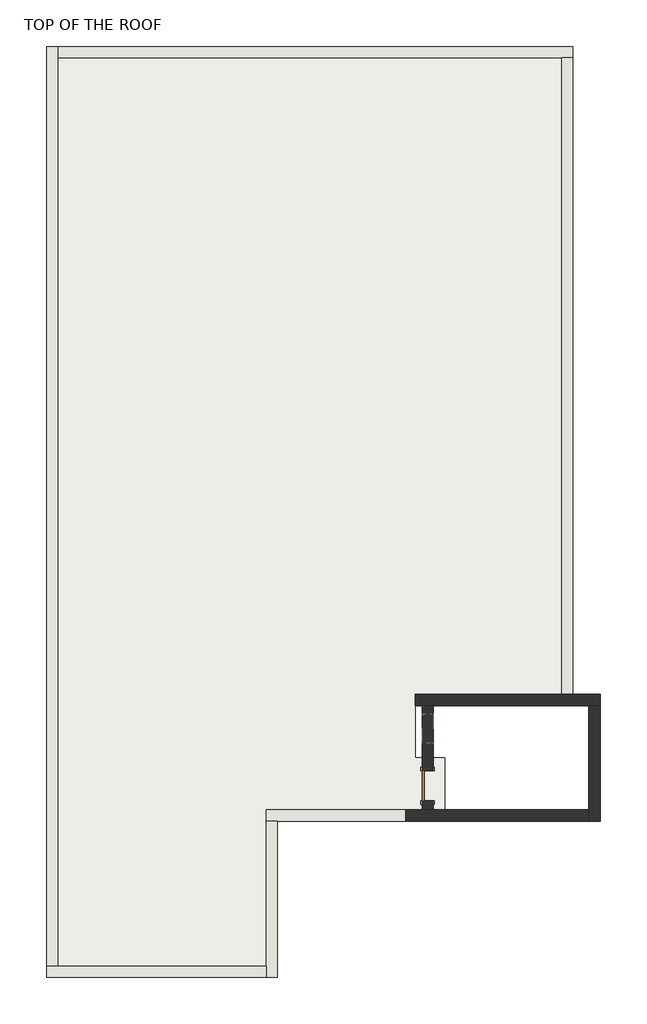
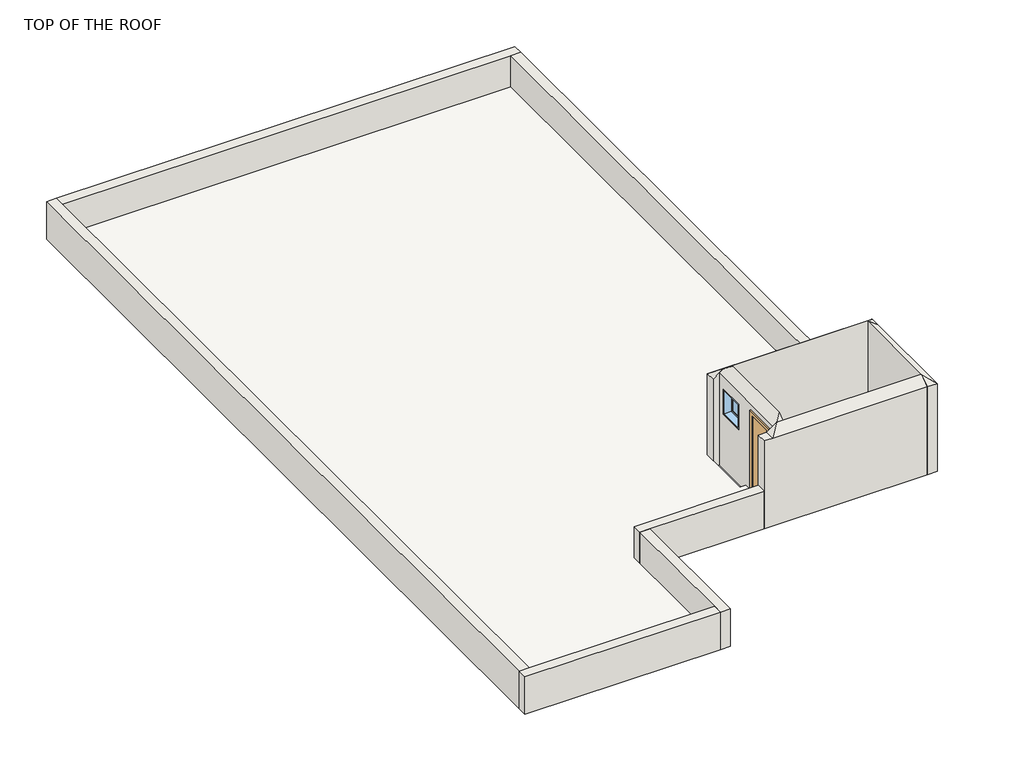
# One storey, incomplete: 10 walls, 1 door, 1 roof, 1 window.
"""IFC4 building model written with IfcOpenShell, lengths in millimetres."""

from ifc_helpers import new_model, si_unit, frame, origin, place, context, project, spatial, polyline, outline, extrude, faceted_brep, transform, mapped, element, save
from components import single_flush_bathroom_flush_door_2_x_7_88cc3d71, window_80340324

model = new_model("IFC4")

# Units and contexts
model_context = context("Model", 3, world=origin())
ifc_project = project(units=[si_unit("LENGTHUNIT", "METRE", prefix="MILLI")], contexts=[model_context])

# Site, building, storey
site = spatial("IfcSite", under=ifc_project)
building = spatial("IfcBuilding", under=site)
storey = spatial("IfcBuildingStorey", under=building, Name="TOP OF THE ROOF", Elevation=6400.8)

# Door
placement = place(None, origin())
single_flush_bathroom_flush_door_2_x_7_shape = single_flush_bathroom_flush_door_2_x_7_88cc3d71(model_context)
element("IfcDoor", 1, ObjectType="Single-Flush : BATHROOM FLUSH DOOR 2' X 7'", at=placement, inside=storey, context=model_context, shape_type="MappedRepresentation", body=[
    mapped(single_flush_bathroom_flush_door_2_x_7_shape, transform((-12501.7436606, -3516.6024127, 6400.8), x_axis=(0.0, 1.0, 0.0), y_axis=(-1.0, 0.0, 0.0), z_axis=(0.0, 0.0, 1.0))),
])

# Roof
element("IfcRoof", 2, ObjectType="Generic - 12\"", at=placement, inside=storey, context=model_context, shape_type="SweptSolid", body=[
    extrude(outline(polyline([(-20070.9436606, 11380.4975873), (-9758.5436606, 11380.4975873), (-9758.5436606, -1649.7024127), (-12755.7436606, -1649.7024127), (-12755.7436606, -1878.3024127), (-12755.7436606, -2945.1024127), (-12146.1436606, -2945.1024127), (-12146.1436606, -4011.9024127), (-15803.7436606, -4011.9024127), (-15803.7436606, -7212.3024127), (-20070.9436606, -7212.3024127), (-20070.9436606, 11380.4975873)])), frame((0.0, 0.0, 6400.8), z_axis=(0.0, 0.0, 1.0), x_axis=(1.0, 0.0, 0.0)), (0.0, 0.0, 1.0), 152.4),
])

# Walls
element("IfcWall", 3, at=placement, inside=storey, context=model_context, shape_type="Brep", body=[
    faceted_brep([(-12755.7436606, -1878.3024127, 6400.8), (-12616.0436606, -1878.3024127, 6400.8), (-12387.4436606, -1878.3024127, 6400.8), (-9199.7436606, -1878.3024127, 6400.8), (-8971.1436606, -1878.3024127, 6400.8), (-8971.1436606, -1878.3024127, 8534.4), (-9199.7436606, -1878.3024127, 8705.85), (-12387.4436606, -1878.3024127, 8705.85), (-12527.1436606, -1878.3024127, 8705.85), (-12616.0436606, -1878.3024127, 8639.175), (-12755.7436606, -1878.3024127, 8534.4), (-12755.7436606, -1649.7024127, 6400.8), (-12755.7436606, -1649.7024127, 8534.4), (-8971.1436606, -1649.7024127, 8534.4), (-8971.1436606, -1649.7024127, 6400.8), (-9529.9436606, -1649.7024127, 6400.8), (-9758.5436606, -1649.7024127, 6400.8)], [[[0, 1, 2, 3, 4, 5, 6, 7, 8, 9, 10]], [[11, 12, 13, 14, 15, 16]], [[4, 3, 2, 1, 0, 11, 16, 15, 14]], [[0, 10, 12, 11]], [[5, 4, 14, 13]], [[10, 9, 8, 12]], [[8, 7, 6, 13, 12]], [[6, 5, 13]]]),
])
element("IfcWall", 4, at=placement, inside=storey, context=model_context, shape_type="Brep", body=[
    faceted_brep([(-9199.7436606, -1878.3024127, 6400.8), (-9199.7436606, -4011.9024127, 6400.8), (-9199.7436606, -4240.5024127, 6400.8), (-9199.7436606, -4240.5024127, 8534.4), (-9199.7436606, -4011.9024127, 8705.85), (-9199.7436606, -1878.3024127, 8705.85), (-8971.1436606, -1878.3024127, 6400.8), (-8971.1436606, -1878.3024127, 8534.4), (-8971.1436606, -4240.5024127, 8534.4), (-8971.1436606, -4240.5024127, 6400.8)], [[[0, 1, 2, 3, 4, 5]], [[6, 7, 8, 9]], [[2, 1, 0, 6, 9]], [[0, 5, 7, 6]], [[3, 2, 9, 8]], [[5, 4, 8, 7]], [[4, 3, 8]]]),
])
element("IfcWall", 5, at=placement, inside=storey, context=model_context, shape_type="Brep", body=[
    faceted_brep([(-9199.7436606, -4011.9024127, 6400.8), (-12387.4436606, -4011.9024127, 6400.8), (-12616.0436606, -4011.9024127, 6400.8), (-12946.2436606, -4011.9024127, 6400.8), (-12946.2436606, -4011.9024127, 7315.2), (-12946.2436606, -4011.9024127, 8534.4), (-12755.7436606, -4011.9024127, 8534.4), (-12616.0436606, -4011.9024127, 8639.175), (-12527.1436606, -4011.9024127, 8705.85), (-12387.4436606, -4011.9024127, 8705.85), (-9199.7436606, -4011.9024127, 8705.85), (-9199.7436606, -4240.5024127, 6400.8), (-9199.7436606, -4240.5024127, 8534.4), (-12755.7436606, -4240.5024127, 8534.4), (-12946.2436606, -4240.5024127, 8534.4), (-12946.2436606, -4240.5024127, 7315.2), (-12946.2436606, -4240.5024127, 6400.8)], [[[0, 1, 2, 3, 4, 5, 6, 7, 8, 9, 10]], [[11, 12, 13, 14, 15, 16]], [[3, 2, 1, 0, 11, 16]], [[5, 4, 3, 16, 15, 14]], [[0, 10, 12, 11]], [[6, 5, 14, 13]], [[10, 9, 8, 13, 12]], [[8, 7, 6, 13]]]),
])
element("IfcWall", 6, at=placement, inside=storey, context=model_context, shape_type="Brep", body=[
    faceted_brep([(-12946.2436606, -4011.9024127, 6400.8), (-15803.7436606, -4011.9024127, 6400.8), (-15803.7436606, -4011.9024127, 7315.2), (-12946.2436606, -4011.9024127, 7315.2), (-12946.2436606, -4240.5024127, 6400.8), (-12946.2436606, -4240.5024127, 7315.2), (-15575.1436606, -4240.5024127, 7315.2), (-15803.7436606, -4240.5024127, 7315.2), (-15803.7436606, -4240.5024127, 6400.8), (-15575.1436606, -4240.5024127, 6400.8)], [[[0, 1, 2, 3]], [[4, 5, 6, 7, 8, 9]], [[1, 0, 4, 9, 8]], [[3, 2, 7, 6, 5]], [[0, 3, 5, 4]], [[2, 1, 8, 7]]]),
])
element("IfcWall", 7, at=placement, inside=storey, context=model_context, shape_type="Brep", body=[
    faceted_brep([(-15803.7436606, -4240.5024127, 6400.8), (-15803.7436606, -7212.3024127, 6400.8), (-15803.7436606, -7440.9024127, 6400.8), (-15803.7436606, -7440.9024127, 7315.2), (-15803.7436606, -7212.3024127, 7315.2), (-15803.7436606, -4240.5024127, 7315.2), (-15575.1436606, -4240.5024127, 6400.8), (-15575.1436606, -4240.5024127, 7315.2), (-15575.1436606, -7440.9024127, 7315.2), (-15575.1436606, -7440.9024127, 6400.8)], [[[0, 1, 2, 3, 4, 5]], [[6, 7, 8, 9]], [[2, 1, 0, 6, 9]], [[5, 4, 3, 8, 7]], [[0, 5, 7, 6]], [[3, 2, 9, 8]]]),
])
element("IfcWall", 8, at=placement, inside=storey, context=model_context, shape_type="Brep", body=[
    faceted_brep([(-15803.7436606, -7212.3024127, 6400.8), (-20070.9436606, -7212.3024127, 6400.8), (-20299.5436606, -7212.3024127, 6400.8), (-20299.5436606, -7212.3024127, 7315.2), (-20070.9436606, -7212.3024127, 7315.2), (-15803.7436606, -7212.3024127, 7315.2), (-15803.7436606, -7440.9024127, 6400.8), (-15803.7436606, -7440.9024127, 7315.2), (-20299.5436606, -7440.9024127, 7315.2), (-20299.5436606, -7440.9024127, 6400.8)], [[[0, 1, 2, 3, 4, 5]], [[6, 7, 8, 9]], [[2, 1, 0, 6, 9]], [[5, 4, 3, 8, 7]], [[0, 5, 7, 6]], [[3, 2, 9, 8]]]),
])
element("IfcWall", 9, at=placement, inside=storey, context=model_context, shape_type="Brep", body=[
    faceted_brep([(-20070.9436606, -7212.3024127, 6400.8), (-20070.9436606, 11380.4975873, 6400.8), (-20070.9436606, 11609.0975873, 6400.8), (-20070.9436606, 11609.0975873, 7315.2), (-20070.9436606, 11380.4975873, 7315.2), (-20070.9436606, -7212.3024127, 7315.2), (-20299.5436606, -7212.3024127, 6400.8), (-20299.5436606, -7212.3024127, 7315.2), (-20299.5436606, 11609.0975873, 7315.2), (-20299.5436606, 11609.0975873, 6400.8)], [[[0, 1, 2, 3, 4, 5]], [[6, 7, 8, 9]], [[2, 1, 0, 6, 9]], [[5, 4, 3, 8, 7]], [[0, 5, 7, 6]], [[3, 2, 9, 8]]]),
])
element("IfcWall", 10, at=placement, inside=storey, context=model_context, shape_type="Brep", body=[
    faceted_brep([(-20070.9436606, 11380.4975873, 6400.8), (-9758.5436606, 11380.4975873, 6400.8), (-9529.9436606, 11380.4975873, 6400.8), (-9529.9436606, 11380.4975873, 7315.2), (-9758.5436606, 11380.4975873, 7315.2), (-20070.9436606, 11380.4975873, 7315.2), (-20070.9436606, 11609.0975873, 6400.8), (-20070.9436606, 11609.0975873, 7315.2), (-9529.9436606, 11609.0975873, 7315.2), (-9529.9436606, 11609.0975873, 6400.8)], [[[0, 1, 2, 3, 4, 5]], [[6, 7, 8, 9]], [[2, 1, 0, 6, 9]], [[5, 4, 3, 8, 7]], [[0, 5, 7, 6]], [[3, 2, 9, 8]]]),
])
element("IfcWall", 11, at=placement, inside=storey, context=model_context, shape_type="SweptSolid", body=[
    extrude(outline(polyline([(-9758.5436606, -1649.7024127), (-9758.5436606, 11380.4975873), (-9529.9436606, 11380.4975873), (-9529.9436606, -1649.7024127), (-9758.5436606, -1649.7024127)])), frame((0.0, 0.0, 6400.8), z_axis=(0.0, 0.0, 1.0), x_axis=(1.0, 0.0, 0.0)), (0.0, 0.0, 1.0), 914.4),
])
element("IfcWall", 12, at=placement, inside=storey, context=model_context, shape_type="Brep", body=[
    faceted_brep([(-12616.0436606, -1878.3024127, 6400.8), (-12616.0436606, -3211.8024127, 6400.8), (-12616.0436606, -3211.8024127, 8432.8), (-12616.0436606, -3821.4024127, 8432.8), (-12616.0436606, -3821.4024127, 6400.8), (-12616.0436606, -4011.9024127, 6400.8), (-12616.0436606, -4011.9024127, 8639.175), (-12616.0436606, -1878.3024127, 8639.175), (-12616.0436606, -2653.0024127, 8341.9666379), (-12616.0436606, -2653.0024127, 7732.3666379), (-12616.0436606, -2043.4024127, 7732.3666379), (-12616.0436606, -2043.4024127, 8341.9666379), (-12387.4436606, -3211.8024127, 8432.8), (-12387.4436606, -3211.8024127, 6400.8), (-12387.4436606, -1878.3024127, 6400.8), (-12387.4436606, -1878.3024127, 8705.85), (-12387.4436606, -2018.0024127, 8810.625), (-12387.4436606, -3872.2024127, 8810.625), (-12387.4436606, -4011.9024127, 8705.85), (-12387.4436606, -4011.9024127, 6400.8), (-12387.4436606, -3821.4024127, 6400.8), (-12387.4436606, -3821.4024127, 8432.8), (-12387.4436606, -2653.0024127, 8341.9666379), (-12387.4436606, -2043.4024127, 8341.9666379), (-12387.4436606, -2043.4024127, 7732.3666379), (-12387.4436606, -2653.0024127, 7732.3666379), (-12527.1436606, -1878.3024127, 8705.85), (-12527.1436606, -4011.9024127, 8705.85)], [[[0, 1, 2, 3, 4, 5, 6, 7], [8, 9, 10, 11]], [[12, 13, 14, 15, 16, 17, 18, 19, 20, 21], [22, 23, 24, 25]], [[20, 19, 5, 4]], [[14, 13, 1, 0]], [[0, 7, 26, 15, 14]], [[6, 5, 19, 18, 27]], [[2, 1, 13, 12]], [[3, 2, 12, 21]], [[4, 3, 21, 20]], [[9, 8, 22, 25]], [[10, 9, 25, 24]], [[11, 10, 24, 23]], [[8, 11, 23, 22]], [[7, 6, 27, 17, 16, 26]], [[27, 18, 17]], [[16, 15, 26]]]),
])

# Window
window_shape = window_80340324(model_context)
element("IfcWindow", 13, ObjectType="Fixed : 24\" x 24\"", at=placement, inside=storey, context=model_context, shape_type="MappedRepresentation", body=[
    mapped(window_shape, transform((-12501.7436606, -2386.3024127, 6817.9666379), x_axis=(0.0, -1.0, 0.0), y_axis=(1.0, 0.0, 0.0), z_axis=(0.0, 0.0, 1.0))),
])

save(model, "model.ifc")

# Revit data of these elements
# Type "Single-Flush : BATHROOM FLUSH DOOR 2' X 7'"
#   Type Mark = "8"
#   Construction Type Id = "MDOOR"
#   Assembly Code = "C1020"
#   Analytic Construction = "Metal"
#   Thickness = 0' - 2"
#   Heat Transfer Coefficient (U) = 0.651978 BTU/(h·ft²·°F)
#   Height = 6' - 8"
#   Trim Projection Ext = 0' - 1"
#   Trim Projection Int = 0' - 1"
#   Trim Width = 0' - 3"
#   Width = 2' - 0"
#   Define Thermal Properties by = 1
#   Door Material = Door - Panel
#   Frame Material = Door - Frame
#   Visual Light Transmittance = 0
#   Solar Heat Gain Coefficient = 0
#   Function = (empty or 0)
#   Wall Closure = (empty or 0)
# Type "Generic - 12\""
#   Assembly Code = "B1020"
#   Layers, outside or top first: 0' - 6" "roof material" (function 1)
# Type
#   Assembly Code = "B2010"
#   Layers, outside or top first: 0' - 9" "TERRACOTTA" (function 1)
# Type "Fixed : 24\" x 24\""
#   Type Mark = "3"
#   Construction Type Id = "GSP4R"
#   Assembly Code = "B2020100"
#   Analytic Construction = "1/8 in Pilkington single glazing"
#   Visual Light Transmittance = 0.9
#   Solar Heat Gain Coefficient = 0.78
#   Heat Transfer Coefficient (U) = 0.6496 BTU/(h·ft²·°F)
#   Height = 2' - 0"
#   Default Sill Height = 3' - 0"
#   Width = 2' - 0"
#   Window Inset = 0' - 0 3/4"
#   Define Thermal Properties by = 1
#   Define Thermal Properties by = 1
#   Glass Pane Material = Glass
#   Sash Material = Sash
#   Wall Closure = (empty or 0)
# Element 1 (IfcDoor, "Single-Flush : BATHROOM FLUSH DOOR 2' X 7'")
#   Phase Created = New Construction
#   Materials on its faces: "Door - Frame", "Door - Panel"
# Element 2 (IfcRoof, "Generic - 12\"")
#   built-in parameter 1001705 = 21.5 (stored number, unit not read)
#   built-in parameter 1001710 = 33615
#   Phase Created = New Construction
#   Materials on its faces: "roof material"
# Elements 3, 4, 5, 12 (IfcWall)
#   Top Offset = 0' - 0"
#   Base Offset = 0' - 0"
#   Unconnected Height = 7' - 0"
#   wall height = 7' - 0"
#   Phase Created = New Construction
#   Base Constraint = TOP OF THE ROOF
#   Materials on its faces: "TERRACOTTA"
# Elements 6, 7, 8, 9, 10, 11 (IfcWall)
#   Top Offset = 0' - 0"
#   Base Offset = 0' - 0"
#   Unconnected Height = 3' - 0"
#   wall height = 3' - 0"
#   Phase Created = New Construction
#   Base Constraint = TOP OF THE ROOF
#   Materials on its faces: "TERRACOTTA"
# Element 13 (IfcWindow, "Fixed : 24\" x 24\"")
#   Mark = "29"
#   Phase Created = New Construction
#   Materials on its faces: "Sash", "Glass"
# Materials
#   "Door - Panel": class "Wood", colour RGB 210 159 95, transparency 0, Cost = 0
#   "Door - Frame": colour RGB 118 70 51, transparency 0, Cost = 0
#   "roof material": class "Generic", colour RGB 120 120 120, transparency 0, Cost = 0
#   "TERRACOTTA": class "Generic", colour RGB 190 112 66, transparency 0, Cost = 0
#   "Glass": class "Glass", colour RGB 0 128 192, transparency 0.75, Description = "Soda Lime Glass", Cost = 0
#   "Sash": class "Wood", colour RGB 224 178 126, transparency 0, Cost = 0
